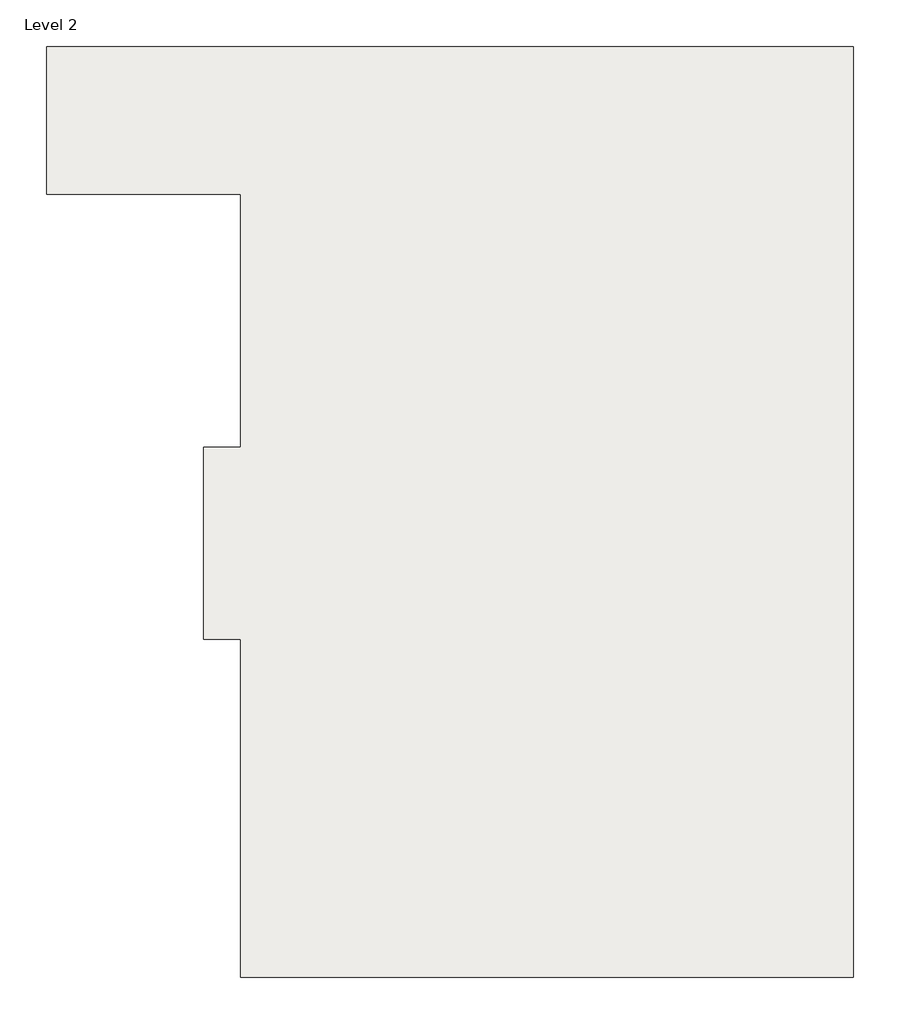
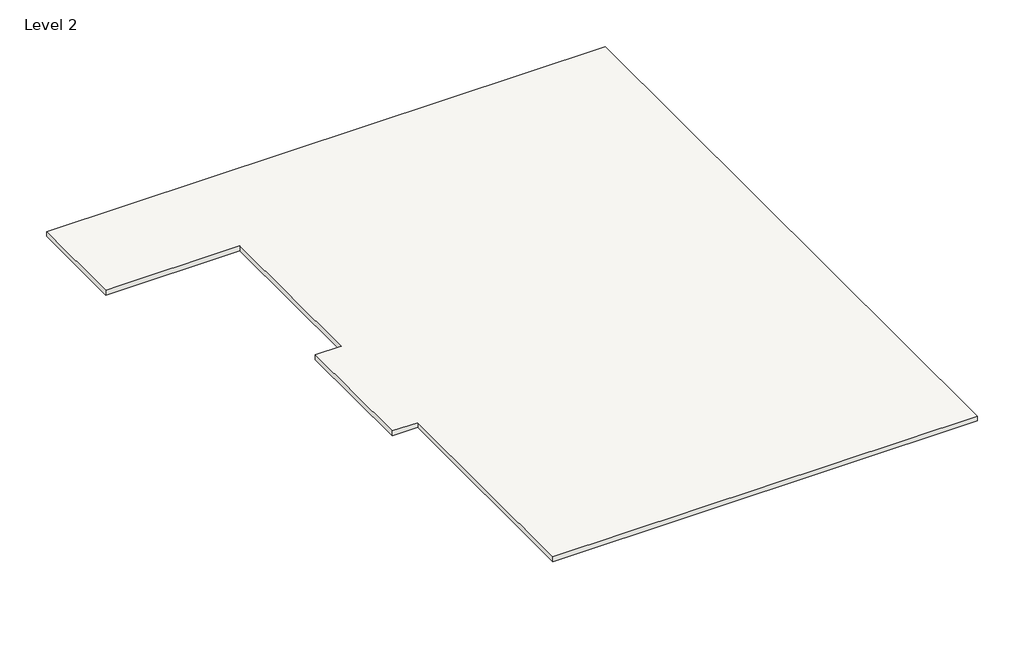
# One storey: 1 roof.
"""IFC4 building model written with IfcOpenShell, lengths in millimetres."""

from ifc_helpers import new_model, si_unit, frame, origin, place, context, project, spatial, polyline, outline, extrude, element, save

model = new_model("IFC4")

# Units and contexts
model_context = context("Model", 3, world=origin())
ifc_project = project(units=[si_unit("LENGTHUNIT", "METRE", prefix="MILLI")], contexts=[model_context])

# Site, building, storey
site = spatial("IfcSite", under=ifc_project)
building = spatial("IfcBuilding", under=site)
storey = spatial("IfcBuildingStorey", under=building, Name="Level 2", Elevation=3048.0)

# Roof
placement = place(None, origin())
element("IfcRoof", 1, ObjectType="Generic - 12\"", at=placement, inside=storey, context=model_context, shape_type="SweptSolid", body=[
    extrude(outline(polyline([(-10241.6673123, 12262.9722985), (6410.607868, 12262.9722985), (6410.607868, -6937.6042186), (-6239.1057305, -6937.6042186), (-6239.1057305, 34.6957814), (-7000.592132, 34.6957814), (-7000.592132, 3997.0957814), (-6238.592132, 3997.0957814), (-6238.592132, 9214.9722985), (-10241.6673123, 9214.9722985), (-10241.6673123, 12262.9722985)])), frame((0.0, 0.0, 3048.0), z_axis=(0.0, 0.0, 1.0), x_axis=(1.0, 0.0, 0.0)), (0.0, 0.0, 1.0), 152.4),
])

save(model, "model.ifc")

# Revit data of these elements
# Type "Generic - 12\""
#   Assembly Code = "B1020"
#   Layers, outside or top first: 0' - 6" no material (function 1)
# Element 1 (IfcRoof, "Generic - 12\"")
#   built-in parameter 1001705 = 10.5 (stored number, unit not read)
#   built-in parameter 1001710 = 33615
#   Phase Created = New Construction
#   Materials on its faces: "Default Roof"
# Materials
#   "Default Roof": colour RGB 88 101 114, transparency 0, Cost = 0
